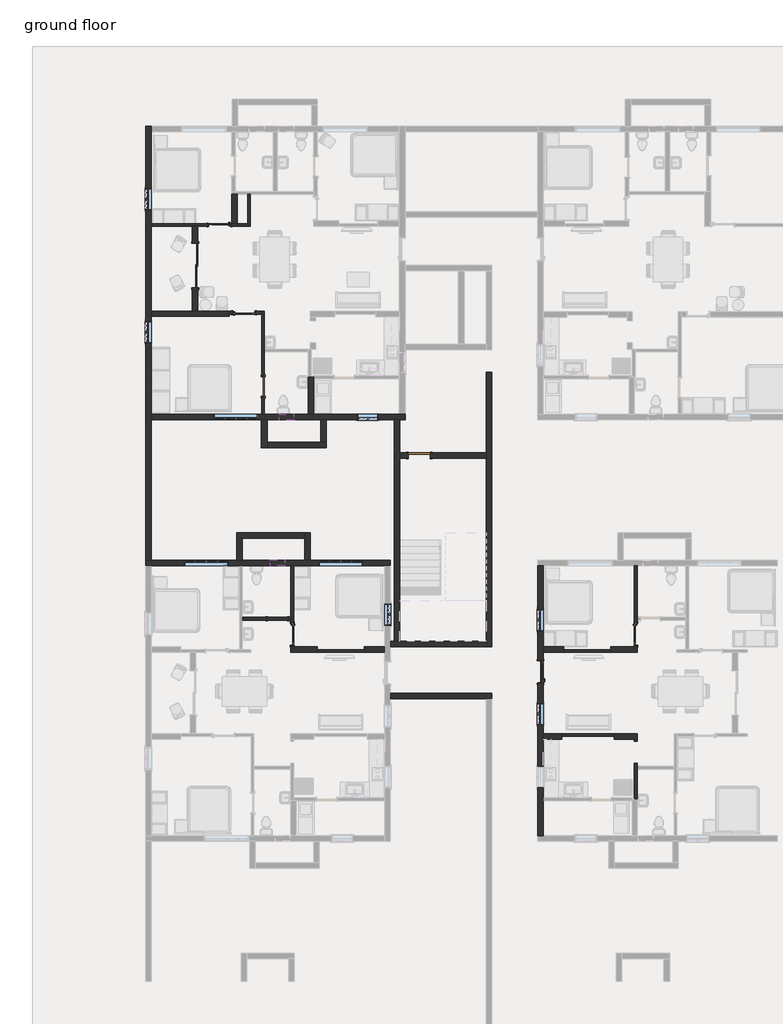
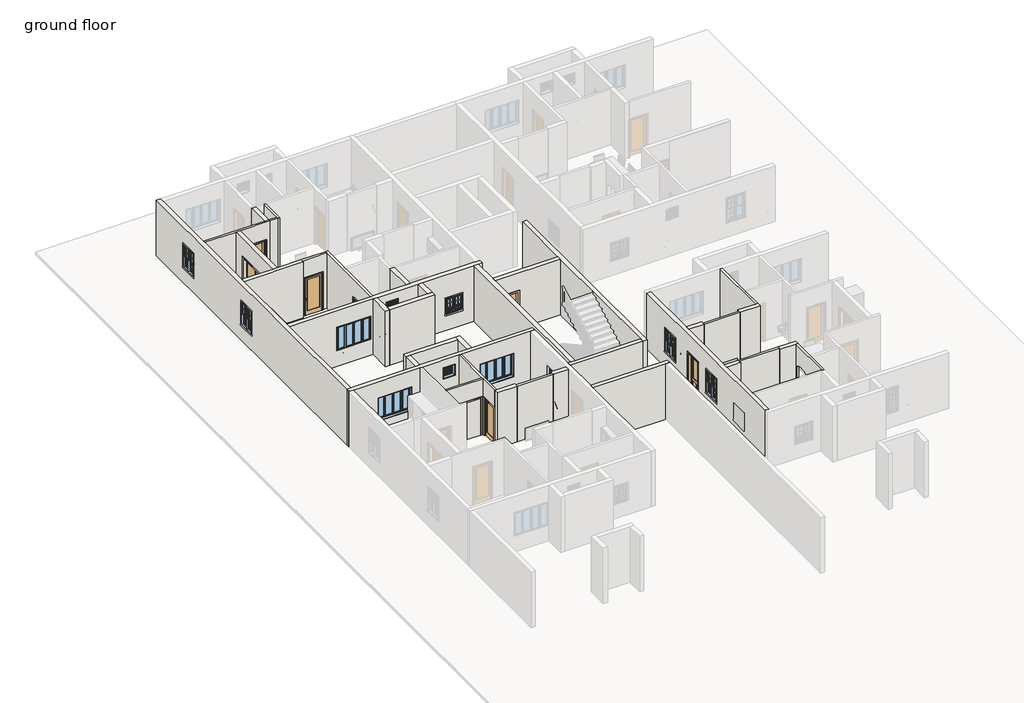
# One storey, part 7 of 16: 38 walls, 11 windows, 9 doors.
# Revit data of these elements (continued)
# Type "Window-Single-Hung-Double : 36\" x 52\"" (continued)
#   Interior Wall Closure [instance default] = 0' - 1 1/2"
#   Rough Width = 3' - 0 1/2"
#   Rough Height = 4' - 4 1/2"
#   Frame Extension [instance default] = 0' - 1 1/4"
#   Exterior Wall Closure [instance default] = 0' - 0 1/2"
#   Extension Jamb [instance default] = 0' - 1 1/2"
#   Heat Transfer Coefficient (U) = 0.5511 BTU/(h·ft²·°F)
#   Height = 4' - 4"
#   Width = 3' - 0"
#   Top Muntin Visibility = yes
#   Indicator Visibility [instance default] = yes
#   Extension Jamb Visibility [instance default] = yes
#   Interior Trim Visibility [instance default] = yes
#   Exterior Trim Visibility [instance default] = yes
#   Define Thermal Properties by = 1
#   Bottom Muntin Visibility = yes
#   Muntin Pattern = Muntin Pattern_2x2 : Muntin Pattern_2x2
#   Interior Trim = Trim-Window-Interior-Flat : Picture Frame
#   Interior Trim Material = Wood - Stained
#   Exterior Trim Material = Clad - White
#   Exterior Trim = Trim-Window-Exterior-Flat : with Sill
#   Glass Panel Material = Glass
#   Exterior Frame Material = Clad - White
#   Interior Frame Material = Wood - Stained
#   Wall Closure = (empty or 0)
# Element 1 (IfcDoor, "36\" x 84\"")
#   Threshold Offset = 0' - 0 1/2"
#   Swing Angle = 90.00°
#   Door Offset = 0' - 0"
#   Threshold = yes
#   Exterior Trim = yes
#   Phase Created = New Construction
#   Materials on its faces: "Cherry", "Aluminum", "Glass"
# Element 2 (IfcDoor, "Door-Double-Sliding : 72\" x 84\"")
#   Phase Created = New Construction
#   Materials on its faces: "Paint - Sienna", "Wood - Birch - Solid Stained Light Low Gloss", "Glass"
# Elements 3, 4, 5, 6 (IfcDoor, "Door-Interior-Single-1_Panel-Wood : 36\" x 84\"")
#   Swing Angle = 90.00°
#   Phase Created = New Construction
#   Materials on its faces: "Cherry", "Aluminum"
# Elements 7, 8 (IfcDoor, "Single-Flush : 32\" x 84\"")
#   Phase Created = New Construction
#   Materials on its faces: "Door - Frame", "Door - Panel"
# Element 9 (IfcDoor, "Single-Flush : 36\" x 84\"")
#   Phase Created = New Construction
#   Materials on its faces: "Door - Frame", "Door - Panel"
# Elements 10, 11, 12, 13, 14, 15, 16, 17, 18, 19, 20, 21, 22 (IfcWall, "Generic - 4.5\"")
#   Top Offset = 0' - 0"
#   Base Offset = 0' - 0"
#   wall height = 10' - 6"
#   Phase Created = New Construction
#   Base Constraint = ground floor
#   Top Constraint = 1st floor
#   Materials on its faces: "Default Wall"
# Element 23 (IfcWall, "Generic - 8\"")
#   Top Offset = 0' - 0"
#   Base Offset = 0' - 0"
#   wall height = 10' - 6"
#   Phase Created = New Construction
#   Base Constraint = ground floor
#   Top Constraint = 1st floor
#   Materials on its faces: "Default Wall"
# Elements 24, 25, 26, 27, 28, 29, 30, 31, 32, 33, 34, 35, 36, 37, 38, 39, 40, 41, 42, 43, 44, 45, 46, 47 (IfcWall, "Generic - 9\"")
#   Top Offset = 0' - 0"
#   Base Offset = 0' - 0"
#   wall height = 10' - 6"
#   Phase Created = New Construction
#   Base Constraint = ground floor
#   Top Constraint = 1st floor
#   Materials on its faces: "Default Wall"
# Element 48 (IfcWindow, "Window-Casement-Double-Awning : 34\" x 36\"")
#   Mark = "16"
#   Window Inset = 0' - 0"
#   Interior Wall Closure = 0' - 2 1/4"
#   Frame Extension = 0' - 0 1/4"
#   Exterior Wall Closure = 0' - 1 1/4"
#   Interior Trim Visibility = yes
#   Exterior Trim Visibility = yes
#   Phase Created = New Construction
#   Materials on its faces: "Wood - Stained", "Glass", "Clad - White"
# Element 49 (IfcWindow, "Window-Casement-Multi-Sash-Horizontal : 72\" x 53\"")
#   Mark = "10"
#   Window Inset = 0' - 0 5/8"
#   Frame Gap 3 = 0' - 1 83/128"
#   Frame Gap 2 = 0' - 0 5/8"
#   Phase Created = New Construction
#   Materials on its faces: "Metal - Aluminum", "Glass"
# Element 50 (IfcWindow, "Window-Casement-Multi-Sash-Horizontal : 72\" x 53\"")
#   Mark = "41"
#   Window Inset = 0' - 0 5/8"
#   Frame Gap 3 = 0' - 1 83/128"
#   Frame Gap 2 = 0' - 0 5/8"
#   Phase Created = New Construction
#   Materials on its faces: "Metal - Aluminum", "Glass"
# Element 51 (IfcWindow, "Window-Casement-Multi-Sash-Horizontal : 72\" x 53\"")
#   Mark = "42"
#   Window Inset = 0' - 0 5/8"
#   Frame Gap 3 = 0' - 1 83/128"
#   Frame Gap 2 = 0' - 0 5/8"
#   Phase Created = New Construction
#   Materials on its faces: "Metal - Aluminum", "Glass"
# Element 52 (IfcWindow, "Window-Louvers : 24\" x 24\"")
#   Mark = "3"
#   Blade Width = 1' - 10 1/2"
#   Phase Created = New Construction
#   Materials on its faces: "Birch"
# Element 53 (IfcWindow, "Window-Louvers : 24\" x 24\"")
#   Mark = "111"
#   Blade Width = 1' - 10 1/2"
#   Phase Created = New Construction
#   Materials on its faces: "Birch"
# Element 54 (IfcWindow, "Window-Single-Hung-Double : 36\" x 52\"")
#   Mark = "13"
#   Window Inset = 0' - 0"
#   Interior Wall Closure = 0' - 1 1/2"
#   Frame Extension = 0' - 1 1/4"
#   Exterior Wall Closure = 0' - 0 1/2"
#   Interior Trim Visibility = yes
#   Indicator Visibility = yes
#   Exterior Trim Visibility = yes
#   Phase Created = New Construction
#   Materials on its faces: "Wood - Stained", "Glass", "Clad - White"
# Element 55 (IfcWindow, "Window-Single-Hung-Double : 36\" x 52\"")
#   Mark = "14"
#   Window Inset = 0' - 0"
#   Interior Wall Closure = 0' - 1 1/2"
#   Frame Extension = 0' - 1 1/4"
#   Exterior Wall Closure = 0' - 0 1/2"
#   Interior Trim Visibility = yes
#   Indicator Visibility = yes
#   Exterior Trim Visibility = yes
#   Phase Created = New Construction
#   Materials on its faces: "Wood - Stained", "Glass", "Clad - White"
# Element 56 (IfcWindow, "Window-Single-Hung-Double : 36\" x 52\"")
#   Mark = "46"
#   Window Inset = 0' - 0"
#   Interior Wall Closure = 0' - 1 1/2"
#   Frame Extension = 0' - 1 1/4"
#   Exterior Wall Closure = 0' - 0 1/2"
#   Interior Trim Visibility = yes
#   Indicator Visibility = yes
#   Exterior Trim Visibility = yes
#   Phase Created = New Construction
#   Materials on its faces: "Wood - Stained", "Glass", "Clad - White"
# Element 57 (IfcWindow, "Window-Single-Hung-Double : 36\" x 52\"")
#   Mark = "67"
#   Window Inset = 0' - 0"
#   Interior Wall Closure = 0' - 1 1/2"
#   Frame Extension = 0' - 1 1/4"
#   Exterior Wall Closure = 0' - 0 1/2"
#   Interior Trim Visibility = yes
#   Indicator Visibility = yes
#   Exterior Trim Visibility = yes
#   Phase Created = New Construction
#   Materials on its faces: "Wood - Stained", "Glass", "Clad - White"
# Element 58 (IfcWindow, "Window-Single-Hung-Double : 36\" x 52\"")
#   Mark = "68"
#   Window Inset = 0' - 0"
#   Interior Wall Closure = 0' - 1 1/2"
#   Frame Extension = 0' - 1 1/4"
#   Exterior Wall Closure = 0' - 0 1/2"
#   Interior Trim Visibility = yes
#   Indicator Visibility = yes
#   Exterior Trim Visibility = yes
#   Phase Created = New Construction
#   Materials on its faces: "Wood - Stained", "Glass", "Clad - White"
# Materials
#   "Cherry": class "Wood", colour RGB 226 177 128, transparency 0, Description = "Prunus Serotina", Cost = 0
#   "Glass": class "Glass", colour RGB 0 128 192, transparency 0.75, Description = "Soda Lime Glass", Cost = 0
#   "Aluminum": class "Metal", colour RGB 247 247 247, transparency 0, Description = "Aluminum 6061", Cost = 0
#   "Wood - Birch - Solid Stained Light Low Gloss": class "Wood", colour RGB 210 159 95, transparency 0, Cost = 0
#   "Paint - Sienna": colour RGB 118 70 51, transparency 0, Cost = 0
#   "Door - Panel": class "Wood", colour RGB 210 159 95, transparency 0, Cost = 0
#   "Door - Frame": colour RGB 118 70 51, transparency 0, Cost = 0
#   "Wood - Stained": class "Wood", colour RGB 224 178 126, transparency 0, Cost = 0
#   "Clad - White": class "Wood", colour RGB 242 242 238, transparency 0, Cost = 0
#   "Metal - Aluminum": class "Metal", colour RGB 247 247 247, transparency 0
#   "Birch": class "Wood", colour RGB 224 178 126, transparency 0, Description = "Betula Alleghaniensis", Cost = 0
#   "Default Wall": colour RGB 128 128 128, transparency 0, Cost = 0
